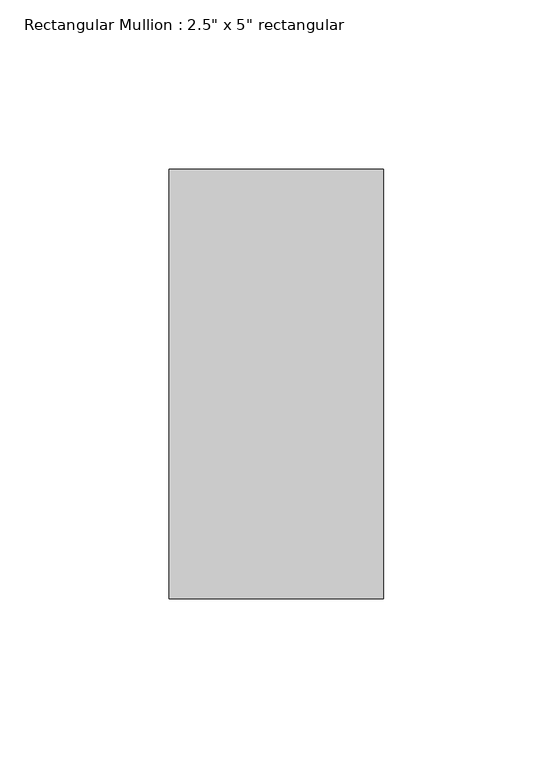
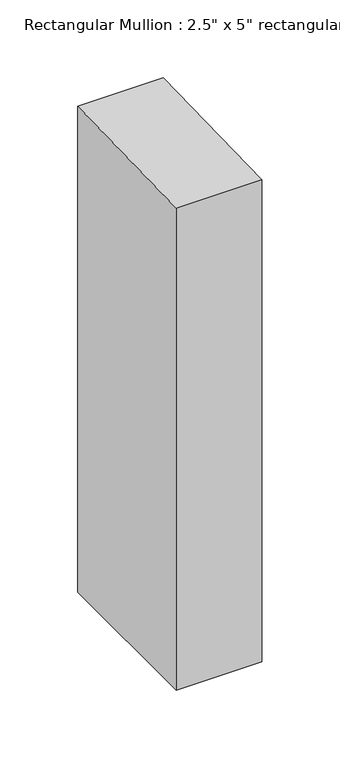
"""IFC4 building model written with IfcOpenShell, lengths in millimetres: member geometry."""

from ifc_helpers import new_model, si_unit, frame, origin, place, context, project, spatial, polyline, outline, extrude, source, transform, mapped, element, save


def member_9a7a48cf(model_context):
    return source(origin(), model_context, "Body", "SweptSolid", [
        extrude(outline(polyline([(-63.5, -1.5241832), (63.5, 1.5241832), (63.5, -380.1195038), (-63.5, -380.1195038), (-63.5, -1.5241832)])), frame((-63.5, 0.0, 0.0), z_axis=(1.0, 0.0, 0.0), x_axis=(0.0, 1.0, 0.0)), (0.0, 0.0, 1.0), 63.5),
    ])


if __name__ == "__main__":
    model = new_model("IFC4")
    model_context = context("Model", 3, world=origin())
    ifc_project = project(units=[si_unit("LENGTHUNIT", "METRE", prefix="MILLI")], contexts=[model_context])
    site = spatial("IfcSite", under=ifc_project)
    building = spatial("IfcBuilding", under=site)
    placement = place(None, origin())
    member_shape = member_9a7a48cf(model_context)
    element("IfcMember", 1, ObjectType="Rectangular Mullion : 2.5\" x 5\" rectangular", at=placement, inside=building, context=model_context, shape_type="MappedRepresentation", body=[
        mapped(member_shape, transform((0.0, 0.0, 0.0), x_axis=(1.0, 0.0, 0.0), y_axis=(0.0, 1.0, 0.0), z_axis=(0.0, 0.0, 1.0))),
    ])
    save(model, "model.ifc")

# Revit data of these elements
# Type "Rectangular Mullion : 2.5\" x 5\" rectangular"
#   built-in parameter 1007304 = 0.416667 (stored number, unit not read)
#   built-in parameter 1007301 = 0.104167 (stored number, unit not read)
#   built-in parameter 1007300 = 0.104167 (stored number, unit not read)
# Element 1 (IfcMember, "Rectangular Mullion : 2.5\" x 5\" rectangular")
#   Materials on its faces: "Aluminum"
# Materials
#   "Aluminum": class "Metal", colour RGB 247 247 247, transparency 0, Description = "Aluminum 6061", Cost = 0
